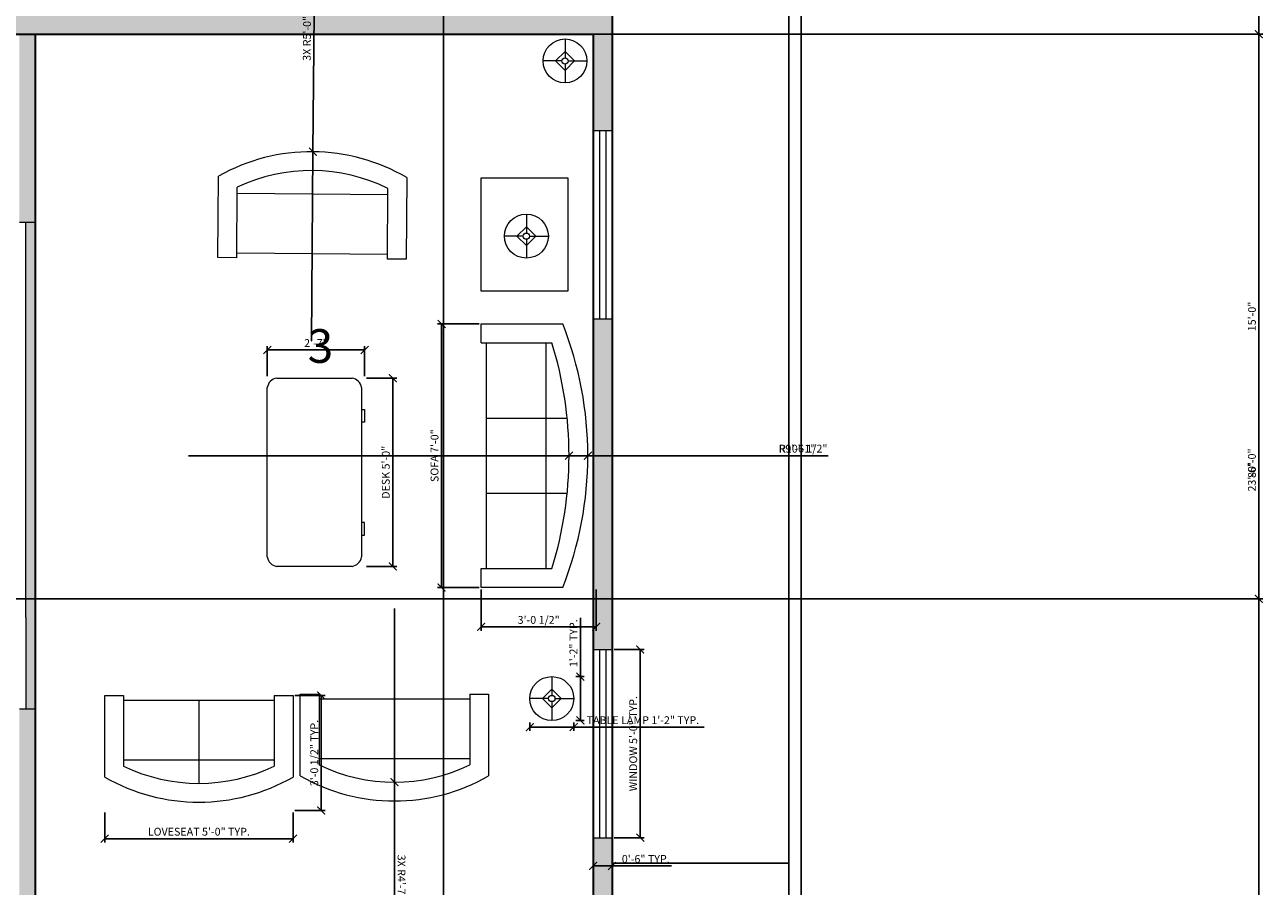
# Model space of a CAD drawing. Units: inches. Extents: x 3122 to 5933, y 1474 to 2995.
# Tile 11 of 12: x 5538 to 5932, y 2261 to 2536. Entities that reach past the tile are written whole.
import ezdxf

# ---------------------------------------------------------------- set-up
doc = ezdxf.new("R2010")
doc.units = ezdxf.units.IN
for name, color, linetype, lineweight in [('A-ANNO-DIMS', 2, 'Continuous', 18), ('A-AREA-IDEN', 7, 'Continuous', 20), ('A-FLOR-STRS', 7, 'Continuous', 25), ('A-FURN', 8, 'Continuous', 18), ('A-GLAZ', 4, 'Continuous', 18), ('A-WALL', 7, 'Continuous', 35), ('A-WALL-PATT', 7, 'Continuous', 13), ('C-PROP', 7, 'Continuous', 25)]:
    doc.layers.add(name, color=color, linetype=linetype, lineweight=lineweight)
doc.styles.get("Standard").update_dxf_attribs({"font": 'arial.ttf'})
doc.dimstyles.new('ISO-25', dxfattribs={"dimtxt": 2.5, "dimasz": 2.5, "dimexe": 1.25, "dimexo": 0.625, "dimtad": 1, "dimdec": 0, "dimlunit": 3, "dimtxsty": 'Standard', "dimblk": 'ARCHTICK', "dimcen": 2.5, "dimadec": 0, "dimazin": 0, "dimtfac": 1, "dimtdec": 0, "dimtmove": 0, "dimatfit": 3, "dimfxl": 1, "dimarcsym": 0})

# ---------------------------------------------------------------- blocks, each defined once
blk = doc.blocks.new('Sofa - Roundback 7 ft.')
for p, q in [((-12.00002, -32.4421), (-12.00003, -6.5971)), ((11.99997, -32.4421), (11.99998, -6.5971)), ((-36.000027, -34), (-36.000027, -11.4696)), ((35.99998, -34), (35.99998, -11.4696)), ((-35.999844, -13.3819), (35.9998, -13.3819)), ((-36.000027, -32.4421), (35.99998, -32.4421))]:
    blk.add_line(p, q)
for points in [[(-36.000027, -34), (-42.000027, -34), (-42.000027, -8)], [(41.99998, -8), (41.99998, -34), (35.99998, -34)]]:
    blk.add_lwpolyline(points)
for centre, radius, start, end in [((0, -114.25), 114.25, 68.43141, 111.5686), ((-0.00001, -127.1968), 121.1968, 72.72033, 107.2797)]:
    blk.add_arc(centre, radius, start, end)
blk = doc.blocks.new('Sofa - Roundback Loveseat 5 ft.')
for p, q in [((0, -32.44198), (0, -5.99998)), ((-24, -33.99998), (-24, -11.46958)), ((24.00004, -33.99998), (24.00004, -11.46958)), ((-23.9998, -13.38178), (23.99986, -13.38178)), ((-24, -32.44198), (24.00004, -32.44198))]:
    blk.add_line(p, q)
for points in [[(-24, -33.99998), (-30, -33.99998), (-30, -7.99998)], [(30.00004, -7.99998), (30.00004, -33.99998), (24.00004, -33.99998)]]:
    blk.add_lwpolyline(points)
for centre, radius, start, end in [((0, -60.24998), 60.24998, 60.13715, 119.8628), ((0, -61.38438), 55.38444, 64.32083, 115.6792)]:
    blk.add_arc(centre, radius, start, end)
blk = doc.blocks.new('Desk - 30 x 60 in.')
for p, q in [((-26.999995, 0), (26.999995, 0)), ((-29.999995, -27), (-29.999995, -3)), ((29.999995, -3), (29.999995, -27)), ((26.999995, -30), (-26.999995, -30)), ((-20.000005, -30), (-20.000005, -31)), ((-20.000005, -31), (-16.000005, -31)), ((-16.000005, -31), (-16.000005, -30)), ((15.999995, -31), (15.999995, -30)), ((19.999995, -31), (15.999995, -31)), ((19.999995, -30), (19.999995, -31))]:
    blk.add_line(p, q)
for centre, start, end in [((-26.499995, -3.5), 98.1301, 171.8699), ((26.499995, -3.5), 8.130102, 81.8699), ((-26.499995, -26.5), 188.1301, 261.8699), ((26.499995, -26.5), 278.1301, 351.8699)]:
    blk.add_arc(centre, 3.535534, start, end)
blk = doc.blocks.new('Lamp - Table')
for p, q in [((0, 7), (0, 1)), ((-1, 0), (-7, 0)), ((0, 3), (-3, 0)), ((-3, 0), (0, -3)), ((3, 0), (0, 3)), ((0, -3), (3, 0)), ((1, 0), (7, 0)), ((0, -1), (0, -7))]:
    blk.add_line(p, q)
for radius in [7, 1]:
    blk.add_circle((0, 0), radius)
blk = doc.blocks.new('WIN-60-DOUBLE-LINE')
for p, q in [((0, 60), (6, 60)), ((2, 60), (2, 0)), ((4, 60), (4, 0)), ((0, 0), (6, 0))]:
    blk.add_line(p, q)
blk = doc.blocks.new('_ArchTick')
at = {"color": 0, "linetype": 'ByBlock', "const_width": 0.15}
blk.add_lwpolyline([(-0.5, -0.5), (0.5, 0.5)], dxfattribs=at)
blk = doc.blocks.new('*D62')
at = {"layer": 'A-ANNO-DIMS', "color": 0, "lineweight": -2, "transparency": 16777216}
for p, q in [((5563.02, 2284.55), (5563.02, 2274.93)), ((5623.02, 2284.55), (5623.02, 2274.93)), ((5623.02, 2276.18), (5563.02, 2276.18))]:
    blk.add_line(p, q, dxfattribs=at)
at = {"layer": 'Defpoints', "color": 0, "transparency": 16777216}
for p in [(5563.02, 2285.18), (5623.02, 2285.18), (5563.02, 2276.18)]:
    blk.add_point(p, dxfattribs=at)
at = {"layer": 'A-ANNO-DIMS', "color": 0, "lineweight": -2, "transparency": 16777216, "xscale": 2.5, "yscale": 2.5, "zscale": 2.5, "rotation": 180}
blk.add_blockref('_ArchTick', (5563.02, 2276.18), dxfattribs=at)
at = {"layer": 'A-ANNO-DIMS', "color": 0, "lineweight": -2, "transparency": 16777216, "xscale": 2.5, "yscale": 2.5, "zscale": 2.5}
blk.add_blockref('_ArchTick', (5623.02, 2276.18), dxfattribs=at)
at = {"layer": 'A-ANNO-DIMS', "color": 0, "transparency": 16777216, "insert": (5593.02, 2278.1), "char_height": 2.5, "attachment_point": 5}
blk.add_mtext('LOVESEAT 5\'-0" TYP.', dxfattribs=at)
blk = doc.blocks.new('*D63')
at = {"layer": 'A-ANNO-DIMS', "color": 0, "lineweight": -2, "transparency": 16777216}
for p, q in [((5623.65, 2321.84), (5633.27, 2321.84)), ((5632.02, 2321.84), (5632.02, 2285.18)), ((5623.65, 2285.18), (5633.27, 2285.18))]:
    blk.add_line(p, q, dxfattribs=at)
at = {"layer": 'Defpoints', "color": 0, "transparency": 16777216}
for p in [(5623.02, 2321.84), (5623.02, 2285.18), (5632.02, 2285.18)]:
    blk.add_point(p, dxfattribs=at)
at = {"layer": 'A-ANNO-DIMS', "color": 0, "lineweight": -2, "transparency": 16777216, "xscale": 2.5, "yscale": 2.5, "zscale": 2.5}
for p, rotation in [((5632.02, 2321.84), 90), ((5632.02, 2285.18), 270)]:
    blk.add_blockref('_ArchTick', p, dxfattribs=dict(at, rotation=rotation))
at = {"layer": 'A-ANNO-DIMS', "color": 0, "transparency": 16777216, "insert": (5630.11, 2303.51), "char_height": 2.5, "attachment_point": 5, "rotation": 90}
blk.add_mtext('3\'-0 1/2" TYP.', dxfattribs=at)
blk = doc.blocks.new('*D68')
at = {"layer": 'A-ANNO-DIMS', "color": 0, "lineweight": -2, "transparency": 16777216}
for p, q in [((5698.46, 2313.25), (5698.46, 2310.53)), ((5712.46, 2313.25), (5712.46, 2310.53)), ((5698.46, 2311.78), (5712.46, 2311.78)), ((5712.46, 2311.78), (5754.03, 2311.78))]:
    blk.add_line(p, q, dxfattribs=at)
at = {"layer": 'Defpoints', "color": 0, "transparency": 16777216}
for p in [(5698.46, 2313.88), (5712.46, 2313.88), (5712.46, 2311.78)]:
    blk.add_point(p, dxfattribs=at)
at = {"layer": 'A-ANNO-DIMS', "color": 0, "lineweight": -2, "transparency": 16777216, "xscale": 2.5, "yscale": 2.5, "zscale": 2.5, "rotation": 180}
blk.add_blockref('_ArchTick', (5698.46, 2311.78), dxfattribs=at)
at = {"layer": 'A-ANNO-DIMS', "color": 0, "lineweight": -2, "transparency": 16777216, "xscale": 2.5, "yscale": 2.5, "zscale": 2.5}
blk.add_blockref('_ArchTick', (5712.46, 2311.78), dxfattribs=at)
at = {"layer": 'A-ANNO-DIMS', "color": 0, "transparency": 16777216, "insert": (5734.49, 2313.66), "char_height": 2.5, "attachment_point": 5}
blk.add_mtext('TABLE LAMP 1\'-2" TYP.', dxfattribs=at)
blk = doc.blocks.new('*D69')
at = {"layer": 'A-ANNO-DIMS', "color": 0, "lineweight": -2, "transparency": 16777216}
for p, q in [((5714.56, 2327.88), (5714.56, 2346.63)), ((5713.08, 2327.88), (5715.81, 2327.88)), ((5714.56, 2313.88), (5714.56, 2327.88)), ((5713.08, 2313.88), (5715.81, 2313.88))]:
    blk.add_line(p, q, dxfattribs=at)
at = {"layer": 'Defpoints', "color": 0, "transparency": 16777216}
for p in [(5712.46, 2327.88), (5714.56, 2327.88), (5712.46, 2313.88)]:
    blk.add_point(p, dxfattribs=at)
at = {"layer": 'A-ANNO-DIMS', "color": 0, "lineweight": -2, "transparency": 16777216, "xscale": 2.5, "yscale": 2.5, "zscale": 2.5}
for p, rotation in [((5714.56, 2327.88), 90), ((5714.56, 2313.88), 270)]:
    blk.add_blockref('_ArchTick', p, dxfattribs=dict(at, rotation=rotation))
at = {"layer": 'A-ANNO-DIMS', "color": 0, "transparency": 16777216, "insert": (5712.68, 2338.51), "char_height": 2.5, "attachment_point": 5, "rotation": 90}
blk.add_mtext('1\'-2" TYP.', dxfattribs=at)
blk = doc.blocks.new('*D74')
at = {"layer": 'A-ANNO-DIMS', "color": 0, "lineweight": -2, "transparency": 16777216}
for p, q in [((5725.28, 2336.51), (5734.9, 2336.51)), ((5733.65, 2276.51), (5733.65, 2336.51)), ((5725.28, 2276.51), (5734.9, 2276.51))]:
    blk.add_line(p, q, dxfattribs=at)
at = {"layer": 'Defpoints', "color": 0, "transparency": 16777216}
for p in [(5724.65, 2336.51), (5733.65, 2336.51), (5724.65, 2276.51)]:
    blk.add_point(p, dxfattribs=at)
at = {"layer": 'A-ANNO-DIMS', "color": 0, "lineweight": -2, "transparency": 16777216, "xscale": 2.5, "yscale": 2.5, "zscale": 2.5}
for p, rotation in [((5733.65, 2336.51), 90), ((5733.65, 2276.51), 270)]:
    blk.add_blockref('_ArchTick', p, dxfattribs=dict(at, rotation=rotation))
at = {"layer": 'A-ANNO-DIMS', "color": 0, "transparency": 16777216, "insert": (5731.73, 2306.51), "char_height": 2.5, "attachment_point": 5, "rotation": 90}
blk.add_mtext('WINDOW 5\'-0" TYP.', dxfattribs=at)
blk = doc.blocks.new('*D75')
at = {"layer": 'A-ANNO-DIMS', "color": 0, "lineweight": -2, "transparency": 16777216}
for p, q in [((5718.65, 2275.88), (5718.65, 2266.26)), ((5724.65, 2275.88), (5724.65, 2266.26)), ((5718.65, 2267.51), (5724.65, 2267.51)), ((5724.65, 2267.51), (5743.64, 2267.51))]:
    blk.add_line(p, q, dxfattribs=at)
at = {"layer": 'Defpoints', "color": 0, "transparency": 16777216}
for p in [(5718.65, 2276.51), (5724.65, 2276.51), (5724.65, 2267.51)]:
    blk.add_point(p, dxfattribs=at)
at = {"layer": 'A-ANNO-DIMS', "color": 0, "lineweight": -2, "transparency": 16777216, "xscale": 2.5, "yscale": 2.5, "zscale": 2.5, "rotation": 180}
blk.add_blockref('_ArchTick', (5718.65, 2267.51), dxfattribs=at)
at = {"layer": 'A-ANNO-DIMS', "color": 0, "lineweight": -2, "transparency": 16777216, "xscale": 2.5, "yscale": 2.5, "zscale": 2.5}
blk.add_blockref('_ArchTick', (5724.65, 2267.51), dxfattribs=at)
at = {"layer": 'A-ANNO-DIMS', "color": 0, "transparency": 16777216, "insert": (5735.4, 2269.41), "char_height": 2.5, "attachment_point": 5}
blk.add_mtext('0\'-6" TYP.', dxfattribs=at)
blk = doc.blocks.new('*D78')
at = {"layer": 'A-ANNO-DIMS', "color": 0, "lineweight": -2, "transparency": 16777216}
for p, q in [((5682.32, 2440.3), (5669.1, 2440.3)), ((5670.35, 2440.3), (5670.35, 2356.3)), ((5682.32, 2356.3), (5669.1, 2356.3))]:
    blk.add_line(p, q, dxfattribs=at)
at = {"layer": 'Defpoints', "color": 0, "transparency": 16777216}
for p in [(5682.95, 2440.3), (5670.35, 2356.3), (5682.95, 2356.3)]:
    blk.add_point(p, dxfattribs=at)
at = {"layer": 'A-ANNO-DIMS', "color": 0, "lineweight": -2, "transparency": 16777216, "xscale": 2.5, "yscale": 2.5, "zscale": 2.5}
for p, rotation in [((5670.35, 2440.3), 90), ((5670.35, 2356.3), 270)]:
    blk.add_blockref('_ArchTick', p, dxfattribs=dict(at, rotation=rotation))
at = {"layer": 'A-ANNO-DIMS', "color": 0, "transparency": 16777216, "insert": (5668.43, 2398.3), "char_height": 2.5, "attachment_point": 5, "rotation": 90}
blk.add_mtext('SOFA 7\'-0"', dxfattribs=at)
blk = doc.blocks.new('*D79')
at = {"layer": 'A-ANNO-DIMS', "color": 0, "lineweight": -2, "transparency": 16777216}
for p, q in [((5682.95, 2355.68), (5682.95, 2342.45)), ((5719.61, 2355.68), (5719.61, 2342.45)), ((5682.95, 2343.7), (5719.61, 2343.7))]:
    blk.add_line(p, q, dxfattribs=at)
at = {"layer": 'Defpoints', "color": 0, "transparency": 16777216}
for p in [(5682.95, 2356.3), (5719.61, 2356.3), (5719.61, 2343.7)]:
    blk.add_point(p, dxfattribs=at)
at = {"layer": 'A-ANNO-DIMS', "color": 0, "lineweight": -2, "transparency": 16777216, "xscale": 2.5, "yscale": 2.5, "zscale": 2.5, "rotation": 180}
blk.add_blockref('_ArchTick', (5682.95, 2343.7), dxfattribs=at)
at = {"layer": 'A-ANNO-DIMS', "color": 0, "lineweight": -2, "transparency": 16777216, "xscale": 2.5, "yscale": 2.5, "zscale": 2.5}
blk.add_blockref('_ArchTick', (5719.61, 2343.7), dxfattribs=at)
at = {"layer": 'A-ANNO-DIMS', "color": 0, "transparency": 16777216, "insert": (5701.28, 2345.62), "char_height": 2.5, "attachment_point": 5}
blk.add_mtext('3\'-0 1/2"', dxfattribs=at)
blk = doc.blocks.new('*D80')
at = {"layer": 'A-ANNO-DIMS', "color": 0, "lineweight": -2, "transparency": 16777216}
for p, q in [((5646.44, 2423.01), (5656.07, 2423.01)), ((5654.82, 2363.01), (5654.82, 2423.01)), ((5646.44, 2363.01), (5656.07, 2363.01))]:
    blk.add_line(p, q, dxfattribs=at)
at = {"layer": 'Defpoints', "color": 0, "transparency": 16777216}
for p in [(5645.82, 2423.01), (5654.82, 2423.01), (5645.82, 2363.01)]:
    blk.add_point(p, dxfattribs=at)
at = {"layer": 'A-ANNO-DIMS', "color": 0, "lineweight": -2, "transparency": 16777216, "xscale": 2.5, "yscale": 2.5, "zscale": 2.5}
for p, rotation in [((5654.82, 2423.01), 90), ((5654.82, 2363.01), 270)]:
    blk.add_blockref('_ArchTick', p, dxfattribs=dict(at, rotation=rotation))
at = {"layer": 'A-ANNO-DIMS', "color": 0, "transparency": 16777216, "insert": (5652.9, 2393.01), "char_height": 2.5, "attachment_point": 5, "rotation": 90}
blk.add_mtext('DESK 5\'-0"', dxfattribs=at)
blk = doc.blocks.new('*D81')
at = {"layer": 'A-ANNO-DIMS', "color": 0, "lineweight": -2, "transparency": 16777216}
for p, q in [((5614.82, 2423.63), (5614.82, 2433.26)), ((5645.82, 2432.01), (5614.82, 2432.01)), ((5645.82, 2423.63), (5645.82, 2433.26))]:
    blk.add_line(p, q, dxfattribs=at)
at = {"layer": 'Defpoints', "color": 0, "transparency": 16777216}
for p in [(5614.82, 2432.01), (5614.82, 2423.01), (5645.82, 2423.01)]:
    blk.add_point(p, dxfattribs=at)
at = {"layer": 'A-ANNO-DIMS', "color": 0, "lineweight": -2, "transparency": 16777216, "xscale": 2.5, "yscale": 2.5, "zscale": 2.5, "rotation": 180}
blk.add_blockref('_ArchTick', (5614.82, 2432.01), dxfattribs=at)
at = {"layer": 'A-ANNO-DIMS', "color": 0, "lineweight": -2, "transparency": 16777216, "xscale": 2.5, "yscale": 2.5, "zscale": 2.5}
blk.add_blockref('_ArchTick', (5645.82, 2432.01), dxfattribs=at)
at = {"layer": 'A-ANNO-DIMS', "color": 0, "transparency": 16777216, "insert": (5630.32, 2433.89), "char_height": 2.5, "attachment_point": 5}
blk.add_mtext('2\'-7"', dxfattribs=at)
blk = doc.blocks.new('*D93')
at = {"layer": 'A-ANNO-DIMS', "color": 0, "lineweight": -2, "transparency": 16777216}
for p, q in [((5785.59, 2875.9), (5931.98, 2875.9)), ((5930.73, 1915.9), (5930.73, 2875.9)), ((5785.59, 1915.9), (5931.98, 1915.9))]:
    blk.add_line(p, q, dxfattribs=at)
at = {"layer": 'Defpoints', "color": 0, "transparency": 16777216}
for p in [(5784.96, 2875.9), (5930.73, 2875.9), (5784.96, 1915.9)]:
    blk.add_point(p, dxfattribs=at)
at = {"layer": 'A-ANNO-DIMS', "color": 0, "lineweight": -2, "transparency": 16777216, "xscale": 2.5, "yscale": 2.5, "zscale": 2.5}
for p, rotation in [((5930.73, 2875.9), 90), ((5930.73, 1915.9), 270)]:
    blk.add_blockref('_ArchTick', p, dxfattribs=dict(at, rotation=rotation))
at = {"layer": 'A-ANNO-DIMS', "color": 0, "transparency": 16777216, "insert": (5928.83, 2395.9), "char_height": 2.5, "attachment_point": 5, "rotation": 90}
blk.add_mtext('80\'-0"', dxfattribs=at)
blk = doc.blocks.new('*D107')
at = {"layer": 'A-ANNO-DIMS', "color": 0, "lineweight": -2, "transparency": 16777216}
for p, q in [((5719.28, 2532.69), (5931.98, 2532.69)), ((5930.73, 2250.49), (5930.73, 2532.69)), ((5719.28, 2250.49), (5931.98, 2250.49))]:
    blk.add_line(p, q, dxfattribs=at)
at = {"layer": 'Defpoints', "color": 0, "transparency": 16777216}
for p in [(5718.65, 2532.69), (5930.73, 2532.69), (5718.65, 2250.49)]:
    blk.add_point(p, dxfattribs=at)
at = {"layer": 'A-ANNO-DIMS', "color": 0, "lineweight": -2, "transparency": 16777216, "xscale": 2.5, "yscale": 2.5, "zscale": 2.5}
for p, rotation in [((5930.73, 2532.69), 90), ((5930.73, 2250.49), 270)]:
    blk.add_blockref('_ArchTick', p, dxfattribs=dict(at, rotation=rotation))
at = {"layer": 'A-ANNO-DIMS', "color": 0, "transparency": 16777216, "insert": (5928.83, 2391.59), "char_height": 2.5, "attachment_point": 5, "rotation": 90}
blk.add_mtext('23\'-6"', dxfattribs=at)
blk = doc.blocks.new('*D110')
at = {"layer": 'A-ANNO-DIMS', "color": 0, "lineweight": -2, "transparency": 16777216}
for p, q in [((5487.87, 2643.06), (5487.87, 1792.93)), ((5670.96, 2643.06), (5670.96, 1792.93)), ((5487.87, 1794.18), (5670.96, 1794.18))]:
    blk.add_line(p, q, dxfattribs=at)
at = {"layer": 'Defpoints', "color": 0, "transparency": 16777216}
for p in [(5487.87, 2643.69), (5670.96, 2643.69), (5670.96, 1794.18)]:
    blk.add_point(p, dxfattribs=at)
at = {"layer": 'A-ANNO-DIMS', "color": 0, "lineweight": -2, "transparency": 16777216, "xscale": 2.5, "yscale": 2.5, "zscale": 2.5, "rotation": 180}
blk.add_blockref('_ArchTick', (5487.87, 1794.18), dxfattribs=at)
at = {"layer": 'A-ANNO-DIMS', "color": 0, "lineweight": -2, "transparency": 16777216, "xscale": 2.5, "yscale": 2.5, "zscale": 2.5}
blk.add_blockref('_ArchTick', (5670.96, 1794.18), dxfattribs=at)
at = {"layer": 'A-ANNO-DIMS', "color": 0, "transparency": 16777216, "insert": (5579.42, 1796.09), "char_height": 2.5, "attachment_point": 5}
blk.add_mtext('15\'-3"', dxfattribs=at)
blk = doc.blocks.new('*D116')
at = {"layer": 'A-ANNO-DIMS', "color": 0, "lineweight": -2, "transparency": 16777216}
for p, q in [((5218.59, 2532.69), (5931.98, 2532.69)), ((5930.73, 2352.69), (5930.73, 2532.69)), ((5218.59, 2352.69), (5931.98, 2352.69))]:
    blk.add_line(p, q, dxfattribs=at)
at = {"layer": 'Defpoints', "color": 0, "transparency": 16777216}
for p in [(5217.96, 2532.69), (5930.73, 2532.69), (5217.96, 2352.69)]:
    blk.add_point(p, dxfattribs=at)
at = {"layer": 'A-ANNO-DIMS', "color": 0, "lineweight": -2, "transparency": 16777216, "xscale": 2.5, "yscale": 2.5, "zscale": 2.5}
for p, rotation in [((5930.73, 2532.69), 90), ((5930.73, 2352.69), 270)]:
    blk.add_blockref('_ArchTick', p, dxfattribs=dict(at, rotation=rotation))
at = {"layer": 'A-ANNO-DIMS', "color": 0, "transparency": 16777216, "insert": (5928.83, 2442.69), "char_height": 2.5, "attachment_point": 5, "rotation": 90}
blk.add_mtext('15\'-0"', dxfattribs=at)
blk = doc.blocks.new('*D127')
at = {"layer": 'A-ANNO-DIMS', "color": 0, "lineweight": -2, "transparency": 16777216}
for p in [(5589.75, 2398.3), (5789.78, 2398.3)]:
    blk.add_line(p, (5710.95, 2398.3), dxfattribs=at)
at = {"layer": 'Defpoints', "color": 0, "transparency": 16777216}
for p in [(5589.75, 2398.3), (5710.95, 2398.3)]:
    blk.add_point(p, dxfattribs=at)
at = {"layer": 'A-ANNO-DIMS', "color": 0, "lineweight": -2, "transparency": 16777216, "xscale": 2.5, "yscale": 2.5, "zscale": 2.5, "rotation": 180.0000439657442}
blk.add_blockref('_ArchTick', (5710.95, 2398.3), dxfattribs=at)
at = {"layer": 'A-ANNO-DIMS', "color": 0, "transparency": 16777216, "insert": (5783.67, 2400.21), "char_height": 2.5, "attachment_point": 5, "rotation": 0}
blk.add_mtext('R10\'-1"', dxfattribs=at)
blk = doc.blocks.new('*D128')
at = {"layer": 'A-ANNO-DIMS', "color": 0, "lineweight": -2, "transparency": 16777216}
for p in [(5602.7, 2398.3), (5793.55, 2398.3)]:
    blk.add_line(p, (5716.95, 2398.3), dxfattribs=at)
at = {"layer": 'Defpoints', "color": 0, "transparency": 16777216}
for p in [(5602.7, 2398.3), (5716.95, 2398.3)]:
    blk.add_point(p, dxfattribs=at)
at = {"layer": 'A-ANNO-DIMS', "color": 0, "lineweight": -2, "transparency": 16777216, "xscale": 2.5, "yscale": 2.5, "zscale": 2.5, "rotation": 180.0000516539632}
blk.add_blockref('_ArchTick', (5716.95, 2398.3), dxfattribs=at)
at = {"layer": 'A-ANNO-DIMS', "color": 0, "transparency": 16777216, "insert": (5785.5, 2400.22), "char_height": 2.5, "attachment_point": 5, "rotation": 0.0001}
blk.add_mtext('R9\'-6 1/2"', dxfattribs=at)
blk = doc.blocks.new('*D129')
at = {"layer": 'A-ANNO-DIMS', "color": 0, "lineweight": -2, "transparency": 16777216}
for p in [(5629.75, 2539.17), (5628.86, 2434.94)]:
    blk.add_line(p, (5629.37, 2495.19), dxfattribs=at)
at = {"layer": 'Defpoints', "color": 0, "transparency": 16777216}
for p in [(5629.37, 2495.19), (5628.86, 2434.94)]:
    blk.add_point(p, dxfattribs=at)
at = {"layer": 'A-ANNO-DIMS', "color": 0, "lineweight": -2, "transparency": 16777216, "xscale": 2.5, "yscale": 2.5, "zscale": 2.5, "rotation": 269.5135960976001}
blk.add_blockref('_ArchTick', (5629.37, 2495.19), dxfattribs=at)
at = {"layer": 'A-ANNO-DIMS', "color": 0, "transparency": 16777216, "insert": (5627.78, 2531.35), "char_height": 2.5, "attachment_point": 5, "rotation": 89.5136}
blk.add_mtext('3X R5\'-0"', dxfattribs=at)
blk = doc.blocks.new('*D130')
at = {"layer": 'A-ANNO-DIMS', "color": 0, "lineweight": -2, "transparency": 16777216}
for p in [(5655.34, 2349.62), (5655.34, 2250.26)]:
    blk.add_line(p, (5655.34, 2294.23), dxfattribs=at)
at = {"layer": 'Defpoints', "color": 0, "transparency": 16777216}
for p in [(5655.34, 2349.62), (5655.34, 2294.23)]:
    blk.add_point(p, dxfattribs=at)
at = {"layer": 'A-ANNO-DIMS', "color": 0, "lineweight": -2, "transparency": 16777216, "xscale": 2.5, "yscale": 2.5, "zscale": 2.5, "rotation": 90.0004117351408}
blk.add_blockref('_ArchTick', (5655.34, 2294.23), dxfattribs=at)
at = {"layer": 'A-ANNO-DIMS', "color": 0, "transparency": 16777216, "insert": (5657.26, 2261), "char_height": 2.5, "attachment_point": 5, "rotation": 270.0004}
blk.add_mtext('3X R4\'-7 1/2"', dxfattribs=at)

msp = doc.modelspace()

# ---------------------------------------------------------------- hatches: boundary and pattern name
at = {"layer": 'A-WALL-PATT'}
h = msp.add_hatch(color=256, dxfattribs=at)
h.dxf.hatch_style = 1
h.paths.add_polyline_path([(5536.42, 2643.69), (5487.87, 2643.69), (5487.87, 2667.06), (5485.81, 2667.06), (5481.87, 2667.06), (5481.87, 2643.69), (5481.87, 2590.35), (5487.87, 2590.35), (5487.87, 2634.69), (5524.65, 2634.69), (5524.65, 2538.69), (5487.87, 2538.69), (5487.87, 2554.35), (5481.87, 2554.35), (5481.87, 2532.69), (5524.65, 2532.69), (5658.65, 2532.69), (5718.65, 2532.69), (5718.65, 2501.93), (5724.65, 2501.93), (5724.65, 2549.4), (5718.65, 2549.4), (5718.65, 2538.69), (5658.65, 2538.69), (5658.65, 2573.57), (5658.59, 2573.63), (5654.65, 2573.63), (5654.65, 2538.69), (5594.65, 2538.69), (5594.65, 2573.57), (5594.59, 2573.63), (5590.65, 2573.63), (5590.65, 2538.69), (5530.65, 2538.69), (5530.65, 2634.69), (5536.42, 2634.69)])
h.paths.add_polyline_path([(5735.69, 2643.69), (5679.96, 2643.69), (5679.96, 2710.77), (5720.44, 2710.77), (5720.44, 2687.32), (5737.79, 2687.32), (5737.79, 2692.32), (5725.44, 2692.32), (5725.44, 2715.77), (5679.96, 2715.77), (5679.96, 2866.9), (5775.96, 2866.9), (5775.96, 2692.32), (5773.79, 2692.32), (5773.79, 2687.32), (5775.96, 2687.32), (5775.96, 2643.69), (5775.96, 2591.85), (5784.96, 2591.85), (5784.96, 2875.9), (5670.96, 2875.9), (5670.96, 2818.9), (5412.4, 2818.9), (5412.4, 2812.9), (5460.96, 2812.9), (5460.96, 2719.12), (5404.54, 2719.12), (5404.54, 2713.12), (5466.96, 2713.12), (5481.87, 2713.12), (5481.87, 2703.06), (5487.87, 2703.06), (5487.87, 2719.12), (5466.96, 2719.12), (5466.96, 2812.9), (5670.96, 2812.9), (5670.96, 2643.69), (5572.42, 2643.69), (5572.42, 2634.69), (5718.65, 2634.69), (5718.65, 2549.4), (5724.65, 2549.4), (5724.65, 2591.85), (5739.96, 2591.85), (5739.96, 2596.85), (5724.65, 2596.85), (5724.65, 2634.69), (5735.69, 2634.69)])
h.paths.add_polyline_path([(5594.65, 2634.69), (5590.65, 2634.69), (5590.65, 2603.63), (5594.65, 2603.63)], flags=17)
h.paths.add_polyline_path([(5724.65, 2441.93), (5718.65, 2441.93), (5718.65, 2336.51), (5724.65, 2336.51)])
h.paths.add_polyline_path([(5724.65, 2276.51), (5718.65, 2276.51), (5718.65, 2250.49), (5713.26, 2250.49), (5713.26, 2244.39), (5724.65, 2244.39)])
h.paths.add_polyline_path([(5689.26, 2250.49), (5540.87, 2250.49), (5540.87, 2317.46), (5535.87, 2317.46), (5535.87, 2244.39), (5689.26, 2244.39)])
h.paths.add_polyline_path([(5540.87, 2532.69), (5535.87, 2532.69), (5535.87, 2472.78), (5540.87, 2472.78)])
h.paths.add_polyline_path([(5540.87, 2472.78), (5537.87, 2472.78), (5537.87, 2346.69), (5537.87, 2317.46), (5540.87, 2317.46)])

# ---------------------------------------------------------------- linework, layer by layer
at = {"layer": 'A-FLOR-STRS'}
msp.add_line((5724.65, 2268.39), (5780.96, 2268.39), dxfattribs=at)
at = {"layer": 'A-FURN'}
msp.add_lwpolyline([(5682.95, 2486.91), (5710.61, 2486.91), (5710.61, 2450.71), (5682.95, 2450.71)], close=True, dxfattribs=at)
at = {"layer": 'A-GLAZ'}
for p, q in [((5535.87, 2472.78), (5540.87, 2472.78)), ((5537.87, 2346.69), (5537.87, 2472.78)), ((5537.87, 2346.69), (5537.87, 2317.46)), ((5540.87, 2317.46), (5535.87, 2317.46))]:
    msp.add_line(p, q, dxfattribs=at)
at = {"layer": 'A-WALL'}
for p, q in [((5724.65, 2591.85), (5724.65, 2244.39)), ((5524.65, 2532.69), (5658.65, 2532.69)), ((5540.87, 2532.69), (5540.87, 2250.49)), ((5594.65, 2532.69), (5654.65, 2532.69)), ((5658.65, 2532.69), (5718.65, 2532.69)), ((5718.65, 2532.69), (5718.65, 2250.49))]:
    msp.add_line(p, q, dxfattribs=at)
at = {"layer": 'C-PROP'}
for p, q in [((5784.96, 1915.9), (5784.96, 2875.9)), ((5780.96, 2256.39), (5780.96, 2591.85))]:
    msp.add_line(p, q, dxfattribs=at)

# ---------------------------------------------------------------- block references
at = {"layer": 'A-FURN'}
for p in [(5709.67, 2524.15), (5697.37, 2468.29), (5705.46, 2320.88)]:
    msp.add_blockref('Lamp - Table', p, dxfattribs=at)
for name, p, rotation in [('Sofa - Roundback Loveseat 5 ft.', (5629.37, 2495.19), 359.5133986298454), ('Sofa - Roundback 7 ft.', (5716.95, 2398.3), 270), ('Desk - 30 x 60 in.', (5614.82, 2393.01), 90), ('Sofa - Roundback Loveseat 5 ft.', (5593.02, 2287.84), 180), ('Sofa - Roundback Loveseat 5 ft.', (5655.34, 2288.23), 180)]:
    msp.add_blockref(name, p, dxfattribs=dict(at, rotation=rotation))
at = {"layer": 'A-GLAZ'}
for p in [(5718.65, 2441.93), (5718.65, 2276.51)]:
    msp.add_blockref('WIN-60-DOUBLE-LINE', p, dxfattribs=at)

# ---------------------------------------------------------------- texts
at = {"layer": 'A-AREA-IDEN'}
msp.add_text('3', height=10.72, rotation=0.0333, dxfattribs=at).set_placement((5627.7, 2427.91))

# ---------------------------------------------------------------- dimensions: what is measured, and where the dimension line sits
at = {"layer": 'A-ANNO-DIMS'}
for base, p1, p2, angle, picture, middle in [((5930.73, 2875.9), (5784.96, 1915.9), (5784.96, 2875.9), 90, '*D93', (5928.83, 2395.9)), ((5930.73, 2532.69), (5217.96, 2352.69), (5217.96, 2532.69), 90, '*D116', (5928.83, 2442.69)), ((5930.73, 2532.69), (5718.65, 2250.49), (5718.65, 2532.69), 90, '*D107', (5928.83, 2391.59)), ((5614.82, 2432.01), (5645.82, 2423.01), (5614.82, 2423.01), 180, '*D81', (5630.32, 2433.89))]:
    dim = msp.add_linear_dim(base=base, p1=p1, p2=p2, angle=angle, dimstyle='ISO-25', override={"dimdec": 1, "dimlfac": 1, "dimrnd": 0, "dimzin": 1, "dimdsep": 46, "dimlunit": 4, "dimfrac": 2}, dxfattribs=at)
    dim.commit()
    dim.dimension.update_dxf_attribs({"geometry": picture, "text_midpoint": middle})
for base, p1, p2, picture, middle in [((5670.96, 1794.18), (5487.87, 2643.69), (5670.96, 2643.69), '*D110', (5579.42, 1796.09)), ((5719.61, 2343.7), (5682.95, 2356.3), (5719.61, 2356.3), '*D79', (5701.28, 2345.62))]:
    dim = msp.add_linear_dim(base=base, p1=p1, p2=p2, dimstyle='ISO-25', override={"dimdec": 1, "dimlfac": 1, "dimrnd": 0, "dimzin": 1, "dimdsep": 46, "dimlunit": 4, "dimfrac": 2}, dxfattribs=at)
    dim.commit()
    dim.dimension.update_dxf_attribs({"geometry": picture, "text_midpoint": middle})
for center, mpoint, picture, middle in [((5628.8605, 2434.9401), (5629.372, 2495.1879), '*D129', (5629.6789, 2531.3365)), ((5655.34, 2349.62), (5655.34, 2294.23), '*D130', (5655.34, 2261))]:
    dim = msp.add_radius_dim(center=center, mpoint=mpoint, text='3X <>', dimstyle='ISO-25', override={"dimdec": 1, "dimlfac": 1, "dimrnd": 0, "dimzin": 1, "dimdsep": 46, "dimlunit": 4, "dimfrac": 2}, dxfattribs=at)
    dim.commit()
    dim.dimension.update_dxf_attribs({"geometry": picture, "text_midpoint": middle, "dimtype": 164})
for base, p1, p2, angle, text, picture, middle in [((5670.35, 2356.3), (5682.95, 2440.3), (5682.95, 2356.3), 270, 'SOFA <>', '*D78', (5668.43, 2398.3)), ((5654.82, 2423.01), (5645.82, 2363.01), (5645.82, 2423.01), 90, 'DESK <>', '*D80', (5652.9, 2393.01)), ((5714.56, 2327.88), (5712.46, 2313.88), (5712.46, 2327.88), 90, '<> TYP.', '*D69', (5712.68, 2338.51)), ((5733.65, 2336.51), (5724.65, 2276.51), (5724.65, 2336.51), 90, 'WINDOW <> TYP.', '*D74', (5731.73, 2306.51)), ((5632.02, 2285.18), (5623.02, 2321.84), (5623.02, 2285.18), 270, '<> TYP.', '*D63', (5630.11, 2303.51)), ((5563.02, 2276.18), (5623.02, 2285.18), (5563.02, 2285.18), 180, 'LOVESEAT <> TYP.', '*D62', (5593.02, 2278.1))]:
    dim = msp.add_linear_dim(base=base, p1=p1, p2=p2, angle=angle, text=text, dimstyle='ISO-25', override={"dimdec": 1, "dimlfac": 1, "dimrnd": 0, "dimzin": 1, "dimdsep": 46, "dimlunit": 4, "dimfrac": 2}, dxfattribs=at)
    dim.commit()
    dim.dimension.update_dxf_attribs({"geometry": picture, "text_midpoint": middle})
for center, mpoint, picture, middle in [((5602.697131, 2398.303897), (5716.947131, 2398.304), '*D128', (5785.497131, 2398.3040618)), ((5589.75, 2398.3), (5710.95, 2398.3), '*D127', (5783.67, 2398.3))]:
    dim = msp.add_radius_dim(center=center, mpoint=mpoint, dimstyle='ISO-25', override={"dimdec": 1, "dimlfac": 1, "dimrnd": 0, "dimzin": 1, "dimdsep": 46, "dimlunit": 4, "dimfrac": 2}, dxfattribs=at)
    dim.commit()
    dim.dimension.update_dxf_attribs({"geometry": picture, "text_midpoint": middle, "dimtype": 164})
for base, p1, p2, text, picture, middle in [((5712.46, 2311.78), (5698.46, 2313.88), (5712.46, 2313.88), 'TABLE LAMP <> TYP.', '*D68', (5734.49, 2313.66)), ((5724.65, 2267.51), (5718.65, 2276.51), (5724.65, 2276.51), '<> TYP.', '*D75', (5735.4, 2269.41))]:
    dim = msp.add_linear_dim(base=base, p1=p1, p2=p2, text=text, dimstyle='ISO-25', override={"dimdec": 1, "dimlfac": 1, "dimrnd": 0, "dimzin": 1, "dimdsep": 46, "dimlunit": 4, "dimfrac": 2}, dxfattribs=at)
    dim.commit()
    dim.dimension.update_dxf_attribs({"geometry": picture, "text_midpoint": middle})

doc.saveas('drawing.dxf')
